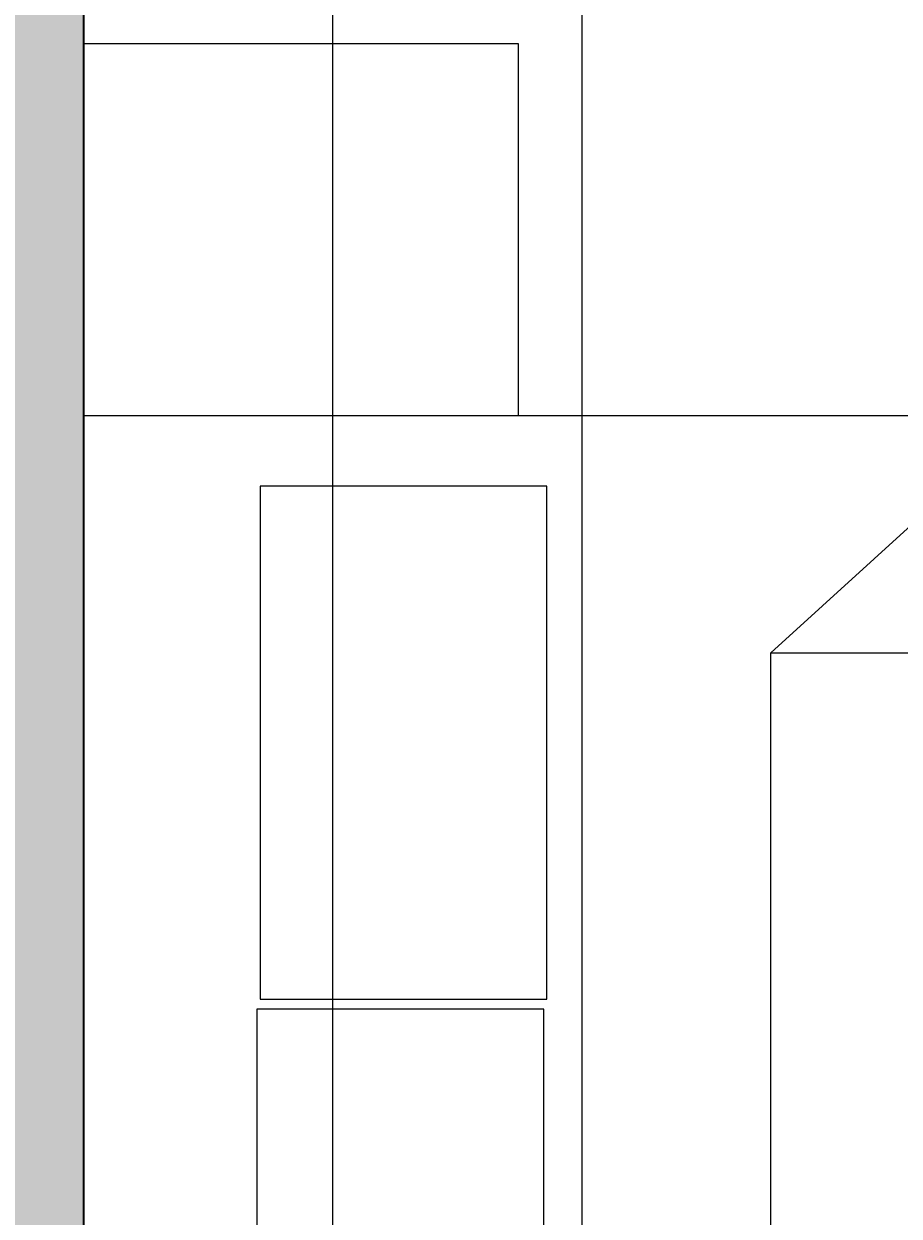
# Model space of a CAD drawing. Units: inches. Extents: x 1998 to 2588, y 1139 to 1977.
# Tile 70 of 134: x 2095 to 2126, y 1817 to 1860. Entities that reach past the tile are written whole.
import ezdxf

# ---------------------------------------------------------------- set-up
doc = ezdxf.new("R2010")
doc.units = ezdxf.units.IN
for name, color, linetype, lineweight in [('A-ANNO-DIMS', 2, 'Continuous', 18), ('A-WALL-PATT', 252, 'Continuous', 13), ('FUR', 21, 'Continuous', 18), ('WALL', 200, 'Continuous', 35)]:
    doc.layers.add(name, color=color, linetype=linetype, lineweight=lineweight)
doc.styles.get("Standard").update_dxf_attribs({"font": 'arial.ttf'})
doc.dimstyles.get("Standard").update_dxf_attribs({"dimtxt": 0.18, "dimasz": 0.18, "dimexe": 0.18, "dimexo": 0.0625, "dimgap": 0.09, "dimtad": 0, "dimtih": 1, "dimtoh": 1, "dimdec": 4, "dimzin": 0, "dimdsep": 46, "dimtxsty": 'Standard', "dimcen": 0.09, "dimadec": 0, "dimazin": 0, "dimtfac": 1, "dimtdec": 4, "dimtofl": 0, "dimtmove": 0, "dimatfit": 3, "dimfxl": 1, "dimtolj": 1, "dimtzin": 0, "dimarcsym": 0})

# ---------------------------------------------------------------- blocks, each defined once
blk = doc.blocks.new('BED-WITH-NIGHTSTANDS')
for p, q in [((34.217, 56), (24.799, 47.436)), ((24.799, 13.424), (24.799, 47.436)), ((24.799, 47.436), (34.217, 47.436))]:
    blk.add_line(p, q)
for points in [[(0, 56), (15.699, 56), (15.699, 69.425), (0, 69.425)], [(0, 56), (65.221, 56), (65.221, 13.424), (0, 13.424)], [(6.374, 34.93), (16.725, 34.93), (16.725, 53.45), (6.374, 53.45)], [(6.254, 16.049), (16.605, 16.049), (16.605, 34.569), (6.254, 34.569)]]:
    blk.add_lwpolyline(points, close=True)
blk = doc.blocks.new('*D40')
at = {"layer": 'A-ANNO-DIMS', "color": 0, "lineweight": -2, "transparency": 16777216}
for p, q in [((2105.973, 1628.541), (2105.973, 1977.362)), ((2106.153, 1977.182), (2110.324, 1977.182)), ((2114.793, 1977.182), (2110.622, 1977.182)), ((2114.973, 1628.804), (2114.973, 1977.362))]:
    blk.add_line(p, q, dxfattribs=at)
at = {"layer": 'A-ANNO-DIMS', "color": 0, "transparency": 16777216}
for points in [[(2106.153, 1977.212), (2106.153, 1977.152), (2105.973, 1977.182)], [(2114.793, 1977.212), (2114.793, 1977.152), (2114.973, 1977.182)]]:
    blk.add_solid(points, dxfattribs=at)
at = {"layer": 'Defpoints', "color": 0, "transparency": 16777216}
for p in [(2114.973, 1977.182), (2105.973, 1628.478), (2114.973, 1628.742)]:
    blk.add_point(p, dxfattribs=at)
at = {"layer": 'A-ANNO-DIMS', "color": 0, "transparency": 16777216, "insert": (2110.473, 1977.182), "char_height": 0.18, "attachment_point": 5}
blk.add_mtext('\\A1;9', dxfattribs=at)

msp = doc.modelspace()

# ---------------------------------------------------------------- hatches: boundary and pattern name
at = {"layer": 'A-WALL-PATT'}
h = msp.add_hatch(color=256, dxfattribs=at)
h.dxf.hatch_style = 1
h.paths.add_polyline_path([(2222.9729, 1888.7324), (2099.4125, 1888.7324), (2099.4125, 1879.7324), (2222.9729, 1879.7324)])
h.paths.add_polyline_path([(2096.9729, 1868.3278), (2087.9729, 1868.3278), (2087.9729, 1775.637), (2096.9729, 1775.637)])
h.paths.add_polyline_path([(2227.4729, 1868.3278), (2222.9729, 1868.3278), (2222.9729, 1774.3318), (2227.4729, 1774.3318)])
h.paths.add_polyline_path([(2188.3019, 1759.7324), (2138.6074, 1759.7324), (2099.4125, 1759.7324), (2099.4125, 1755.2324), (2176.9729, 1755.2324), (2188.3019, 1755.2324)])
h.paths.add_polyline_path([(2087.9729, 1759.7324), (2059.4729, 1759.7324), (2059.4729, 1702.7324), (2087.9729, 1702.7324), (2087.9729, 1707.2324), (2063.9729, 1707.2324), (2063.9729, 1755.2324), (2087.9729, 1755.2324)])
h.paths.add_polyline_path([(2096.9729, 1755.2324), (2087.9729, 1755.2324), (2087.9729, 1707.2324), (2096.9729, 1707.2324)])
h.paths.add_polyline_path([(2187.0461, 1707.2324), (2105.9729, 1707.2324), (2096.9729, 1707.2324), (2087.9729, 1707.2324), (2087.9729, 1702.7324), (2105.9729, 1702.7324), (2114.9729, 1702.7324), (2187.0461, 1702.7324)])
h.paths.add_polyline_path([(2181.4729, 1719.2028), (2176.9729, 1719.2028), (2176.9729, 1707.2324), (2181.4729, 1707.2324)])
h.paths.add_polyline_path([(2216.0332, 1588.7324), (2114.9729, 1588.7324), (2105.9729, 1588.7324), (2105.9729, 1584.2324), (2216.0332, 1584.2324)])
h.paths.add_polyline_path([(2077.691, 1588.7324), (2061.4729, 1588.7324), (2061.4729, 1584.2324), (2077.691, 1584.2324)])
h.paths.add_polyline_path([(2105.9729, 1588.7324), (2098.0956, 1588.7324), (2098.0956, 1584.2324), (2105.9729, 1584.2324)])
h.paths.add_polyline_path([(2114.9729, 1596.2642), (2110.1012, 1596.2642), (2105.9729, 1596.2642), (2105.9729, 1588.7324), (2114.9729, 1588.7324)])
h.paths.add_polyline_path([(2114.9729, 1584.2324), (2105.9729, 1584.2324), (2105.9729, 1580.249), (2110.1012, 1580.249), (2114.9729, 1580.249)])
h.paths.add_polyline_path([(2114.9729, 1547.7716), (2110.1012, 1547.7716, -0.0318759), (2105.9729, 1548.035), (2105.9729, 1470.2324), (2108.3775, 1470.2324), (2108.3775, 1465.7324), (2186.2943, 1465.7324), (2186.2943, 1470.2324), (2114.9729, 1470.2324)])
h.paths.add_polyline_path([(2227.4729, 1584.2324), (2222.9729, 1584.2324), (2222.9729, 1486.137), (2227.4729, 1486.137)])
h.paths.add_polyline_path([(2295.4138, 1593.2324), (2227.4729, 1593.2324), (2227.4729, 1588.7324), (2295.4138, 1588.7324), (2295.4138, 1591.8729)])
h.paths.add_polyline_path([(2345.9729, 1627.1165), (2341.4729, 1627.1165), (2341.4729, 1593.2324), (2337.2869, 1593.2324), (2337.2869, 1591.8729), (2337.2869, 1588.7324), (2345.9729, 1588.7324)])
h.paths.add_polyline_path([(2291.9729, 1588.7324), (2287.4729, 1588.7324), (2287.4729, 1522.7324), (2291.9729, 1522.7324)])
h.paths.add_polyline_path([(2291.9729, 1522.7324), (2287.4729, 1522.7324), (2227.4729, 1522.7324), (2227.4729, 1518.2324), (2291.9729, 1518.2324)])
h.paths.add_polyline_path([(2295.7347, 1519.5919), (2295.7347, 1522.7324), (2291.9729, 1522.7324), (2291.9729, 1518.2324), (2295.7347, 1518.2324)])
h.paths.add_polyline_path([(2345.9729, 1522.7324), (2337.6078, 1522.7324), (2337.6078, 1519.5919), (2337.6078, 1518.2324), (2341.4729, 1518.2324), (2341.4729, 1488.5616), (2345.9729, 1488.5616)])
h.paths.add_polyline_path([(2345.9729, 1468.1569), (2341.4729, 1468.1569), (2341.4729, 1374.2324), (2227.4729, 1374.2324), (2227.4729, 1369.7324), (2345.9729, 1369.7324)])
h.paths.add_polyline_path([(2345.9729, 1369.7324), (2341.4729, 1369.7324), (2341.4729, 1362.2324), (2345.9729, 1362.2324)])
h.paths.add_polyline_path([(2345.9729, 1317.7324), (2345.9729, 1322.2324), (2341.4729, 1322.2324), (2341.4729, 1285.137), (2345.9729, 1285.137)], flags=17)
h.paths.add_polyline_path([(2356.2096, 1322.2324), (2345.9729, 1322.2324), (2345.9729, 1317.7324), (2356.2096, 1317.7324), (2356.2096, 1319.3088)], flags=17)
h.paths.add_polyline_path([(2393.9729, 1322.2324), (2375.6999, 1322.2324), (2375.6999, 1319.3088, -0.0202458), (2375.636, 1317.7324), (2393.9729, 1317.7324)], flags=17)
h.paths.add_polyline_path([(2398.4729, 1322.2324), (2393.9729, 1322.2324), (2393.9729, 1317.7324), (2393.9729, 1237.7324), (2345.9729, 1237.7324), (2345.9729, 1264.7324), (2341.4729, 1264.7324), (2341.4729, 1228.7324), (2393.9729, 1228.7324), (2482.7412, 1228.7324), (2482.7412, 1237.7324), (2398.4729, 1237.7324), (2398.4729, 1297.1029)])
h.paths.add_polyline_path([(2398.4729, 1362.2324), (2393.9729, 1362.2324), (2393.9729, 1357.7324), (2398.4729, 1357.7324)])
h.paths.add_polyline_path([(2345.9729, 1329.7549), (2341.4729, 1329.7549), (2341.4729, 1322.2324), (2345.9729, 1322.2324)])

# ---------------------------------------------------------------- linework, layer by layer
at = {"layer": 'WALL'}
msp.add_line((2096.9729, 1868.3278), (2096.9729, 1775.637), dxfattribs=at)

# ---------------------------------------------------------------- block references
at = {"layer": 'FUR'}
msp.add_blockref('BED-WITH-NIGHTSTANDS', (2096.973, 1790.045), dxfattribs=at)

# ---------------------------------------------------------------- dimensions: what is measured, and where the dimension line sits
at = {"layer": 'A-ANNO-DIMS'}
dim = msp.add_linear_dim(base=(2114.9729, 1977.1824), p1=(2105.9729, 1628.4781), p2=(2114.9729, 1628.7416), dimstyle='Standard', override={"dimdec": 0, "dimlfac": 1, "dimrnd": 0, "dimzin": 0, "dimdsep": 46, "dimlunit": 2}, dxfattribs=at)
dim.commit()
dim.dimension.update_dxf_attribs({"geometry": '*D40', "text_midpoint": (2110.4729, 1977.1824)})

doc.saveas('drawing.dxf')
